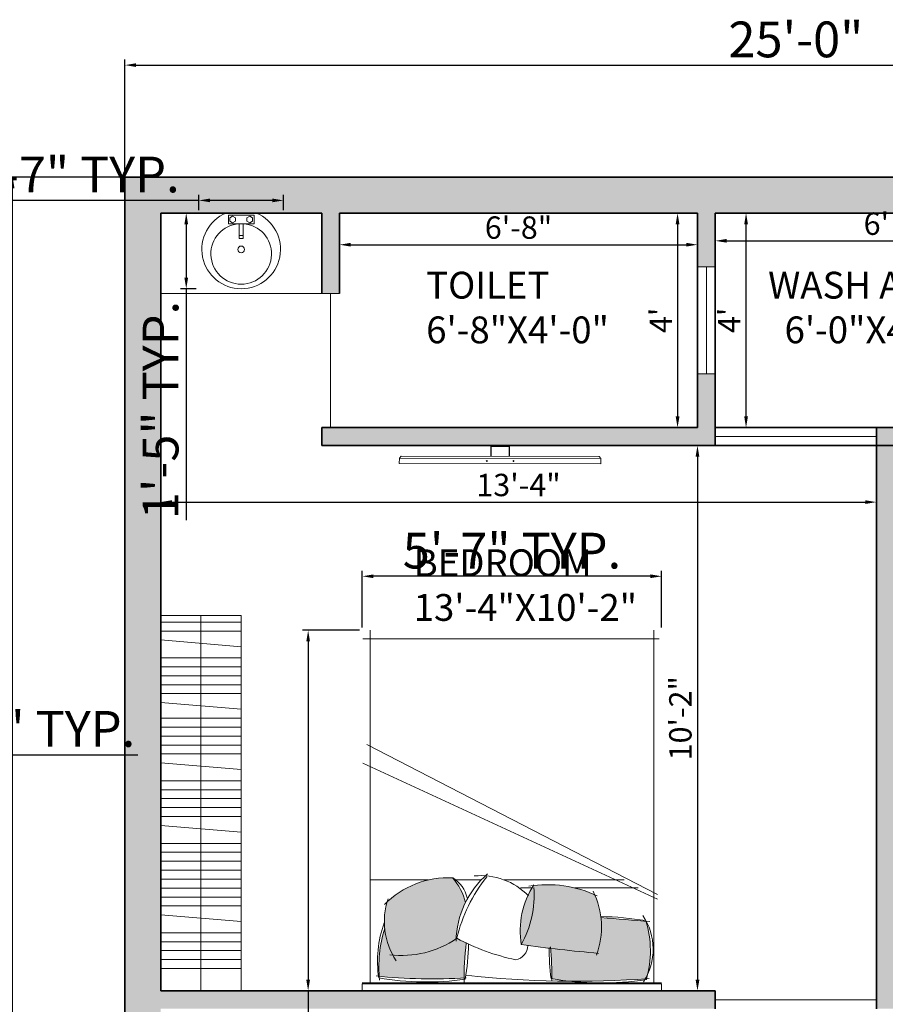
# Model space of a CAD drawing. Units: inches. Extents: x 3259 to 4981, y 1402 to 2026.
# Tile 6 of 11: x 3644 to 3838, y 1722 to 1942. Entities that reach past the tile are written whole.
import ezdxf

# ---------------------------------------------------------------- set-up
doc = ezdxf.new("R2010")
doc.units = ezdxf.units.IN
for name, color, linetype, lineweight in [('0.10', 252, 'Continuous', 9), ('A-ANNO-DIMS', 2, 'Continuous', 13), ('A-AREA-IDEN', 7, 'Continuous', 18), ('A-DOOR', 3, 'Continuous', 18), ('A-EQPM', 8, 'Continuous', 18), ('A-FLOR-CASE', 8, 'Continuous', 18), ('A-FLOR-FIXT', 9, 'Continuous', 18), ('A-FURN', 8, 'Continuous', 13), ('A-GLAZ', 4, 'Continuous', 18), ('A-WALL', 7, 'Continuous', 35), ('A-WALL-PATT', 252, 'Continuous', 13)]:
    doc.layers.add(name, color=color, linetype=linetype, lineweight=lineweight)
doc.layers.add('A-FURN-PATT', color=116, linetype='Continuous', lineweight=13, true_color=0x136734)
doc.styles.get("Standard").update_dxf_attribs({"font": 'arial.ttf'})
doc.dimstyles.new('ISO-25', dxfattribs={"dimtxt": 8, "dimasz": 2.5, "dimexe": 1.25, "dimexo": 0.625, "dimtad": 1, "dimdec": 1, "dimlunit": 3, "dimtxsty": 'Standard', "dimcen": 2.5, "dimclrd": 4, "dimclre": 4, "dimclrt": 1, "dimadec": 0, "dimazin": 0, "dimtfac": 1, "dimtdec": 1, "dimtmove": 0, "dimatfit": 3, "dimfxl": 1, "dimarcsym": 0})

# ---------------------------------------------------------------- blocks, each defined once
blk = doc.blocks.new('camita')
at = {"layer": '0.10'}
for p, q in [((-0.85, -0.045), (0.85, -0.045)), ((-0.805, -0.045), (-0.805, -2.0485)), ((0.805, -0.045), (0.805, -2.0485)), ((-0.8271, -0.521), (0.8464, -1.2932)), ((-0.8271, -0.5476), (0.8236, -1.3992)), ((-0.7161, -0.585), (-0.3554, -0.585)), ((-0.1136, -0.585), (-0.0485, -0.585)), ((-0.638, -0.63), (0.0434, -0.63)), ((0.1749, -0.63), (0.3179, -0.63)), ((0.4739, -0.63), (0.805, -0.63)), ((-0.8354, -2), (0.8464, -2))]:
    blk.add_line(p, q, dxfattribs=at)
blk.add_lwpolyline([(-0.85, -0.0405), (0.85, -0.0405), (0.85, 0), (-0.85, 0)], close=True, dxfattribs=at)
for centre, radius, start, end in [((-0.4574, -0.2364), 0.3443, 147.51, 213.8336), ((-0.3639, -5.8457), 5.7909, 83.80731, 94.12107), ((-0.5104, -1.7232), 1.6781, 80.1255, 98.6619), ((-1.4396, -0.0609), 1.7117, 352.9291, 0.3959), ((0.4863, -1.6286), 1.5781, 80.1602, 98.06), ((-0.1997, -0.2266), 0.5864, 163.9263, 197.1409), ((2.3534, -0.0532), 2.5803, 180.1063, 184.3854), ((-1.5443, -0.2452), 1.3333, 359.9394, 7.5533), ((1.5815, -0.2893), 1.3353, 170.3802, 178.9914), ((0.4524, -3.0675), 2.9996, 83.9026, 93.6759), ((0.0294, -0.1377), 0.7262, 342.5841, 6.0048), ((0.1326, -0.1696), 0.6307, 339.923, 8.7433), ((-0.0543, -0.3633), 0.4542, 159.3026, 206.5026), ((-1.3301, -9.6748), 9.4985, 82.27078, 84.93989), ((-0.007, -0.258), 0.0828, 100.018, 179.736), ((-0.2931, -1.4378), 1.2903, 61.9749, 77.8435), ((0.6265, -0.7518), 0.5508, 82.9691, 124.6739), ((0.3203, -0.3944), 0.4043, 341.4524, 33.4512), ((0.4585, -0.5454), 0.5842, 151.0456, 184.1497), ((-0.5341, -0.3393), 0.4875, 327.2644, 9.0473), ((-0.1986, -0.2742), 0.5159, 310.7395, 359.0576), ((-0.5673, -0.0868), 0.9057, 321.6953, 346.4626), ((-1.8672, -14.986), 14.6323, 84.65974, 85.75157), ((-0.4598, 1.4861), 1.9092, 260.953, 268.6517), ((0.5707, -0.4317), 0.3145, 192.9388, 221.9636), ((0.3612, -0.133), 0.5096, 267.2589, 315.2997), ((-0.2002, 0.064), 0.6673, 244.7809, 279.0606), ((0.179, -0.272), 0.3828, 224.5284, 275.2229), ((0.4384, -0.4834), 0.1898, 193.6849, 236.7035)]:
    blk.add_arc(centre, radius, start, end, dxfattribs=at)
blk = doc.blocks.new('M_BATH_BASIN_Basin - Oval_P')
at = {"color": 0, "linetype": 'ByBlock', "lineweight": -2}
blk.add_lwpolyline([(0, 89.5, -5.027337), (0, -89.5)], format="xyb", close=True, dxfattribs=at)
blk.add_lwpolyline([(63.2, 12, -30), (63.2, -12, -1.097889)], format="xyb", dxfattribs=at)
for points in [[(13.2, -76.2), (13.2, 76.2), (63.2, 76.2), (63.2, -76.2)], [(19.1, 50.8), (28.7, 67.3), (47.7, 67.3), (57.2, 50.8), (47.7, 34.3), (28.7, 34.3)]]:
    blk.add_lwpolyline(points, close=True, dxfattribs=at)
for points in [[(63.2, 12), (151.6, 12), (151.6, -12), (63.2, -12)], [(134.3, 12), (134.3, -12)], [(28.7, -34.3), (47.7, -34.3), (57.2, -50.8), (47.7, -67.3), (28.7, -67.3), (19.1, -50.8), (28.7, -34.3)]]:
    blk.add_lwpolyline(points, dxfattribs=at)
blk.add_circle((216.2, 0), 20.1, dxfattribs=at)
at = {"layer": 'Defpoints'}
for p in [(0, 234), (0, -234)]:
    blk.add_point(p, dxfattribs=at)
blk = doc.blocks.new('*D41')
at = {"layer": 'A-ANNO-DIMS', "color": 0, "lineweight": -2, "transparency": 16777216}
for p, q in [((3715.66, 1898.49), (3715.66, 1890.79)), ((3795.66, 1898.49), (3795.66, 1890.79)), ((3718.16, 1892.04), (3793.16, 1892.04))]:
    blk.add_line(p, q, dxfattribs=at)
at = {"layer": 'A-ANNO-DIMS', "color": 0, "transparency": 16777216}
for points in [[(3718.16, 1892.46), (3718.16, 1891.63), (3715.66, 1892.04)], [(3793.16, 1892.46), (3793.16, 1891.63), (3795.66, 1892.04)]]:
    blk.add_solid(points, dxfattribs=at)
at = {"layer": 'Defpoints', "color": 0, "transparency": 16777216}
for p in [(3715.66, 1899.12), (3795.66, 1899.12), (3795.66, 1892.04)]:
    blk.add_point(p, dxfattribs=at)
at = {"layer": 'A-ANNO-DIMS', "color": 0, "transparency": 16777216, "insert": (3755.66, 1895.22), "char_height": 5, "attachment_point": 5}
blk.add_mtext('6\'-8"', dxfattribs=at)
blk = doc.blocks.new('*D42')
at = {"layer": 'A-ANNO-DIMS', "color": 0, "lineweight": -2, "transparency": 16777216}
for p, q in [((3795.04, 1899.12), (3789.97, 1899.12)), ((3791.22, 1896.62), (3791.22, 1853.62)), ((3795.04, 1851.12), (3789.97, 1851.12))]:
    blk.add_line(p, q, dxfattribs=at)
at = {"layer": 'A-ANNO-DIMS', "color": 0, "transparency": 16777216}
for points in [[(3790.8, 1896.62), (3791.64, 1896.62), (3791.22, 1899.12)], [(3790.8, 1853.62), (3791.64, 1853.62), (3791.22, 1851.12)]]:
    blk.add_solid(points, dxfattribs=at)
at = {"layer": 'Defpoints', "color": 0, "transparency": 16777216}
for p in [(3795.66, 1899.12), (3791.22, 1851.12), (3795.66, 1851.12)]:
    blk.add_point(p, dxfattribs=at)
at = {"layer": 'A-ANNO-DIMS', "color": 0, "transparency": 16777216, "insert": (3788.1, 1875.12), "char_height": 5, "attachment_point": 5, "rotation": 90}
blk.add_mtext("4'", dxfattribs=at)
blk = doc.blocks.new('*D43')
at = {"layer": 'A-ANNO-DIMS', "color": 0, "lineweight": -2, "transparency": 16777216}
for p, q in [((3800.29, 1899.12), (3807.78, 1899.12)), ((3806.53, 1853.62), (3806.53, 1896.62)), ((3800.29, 1851.12), (3807.78, 1851.12))]:
    blk.add_line(p, q, dxfattribs=at)
at = {"layer": 'A-ANNO-DIMS', "color": 0, "transparency": 16777216}
for points in [[(3806.12, 1896.62), (3806.95, 1896.62), (3806.53, 1899.12)], [(3806.12, 1853.62), (3806.95, 1853.62), (3806.53, 1851.12)]]:
    blk.add_solid(points, dxfattribs=at)
at = {"layer": 'Defpoints', "color": 0, "transparency": 16777216}
for p in [(3799.66, 1899.12), (3806.53, 1899.12), (3799.66, 1851.12)]:
    blk.add_point(p, dxfattribs=at)
at = {"layer": 'A-ANNO-DIMS', "color": 0, "transparency": 16777216, "insert": (3803.41, 1875.12), "char_height": 5, "attachment_point": 5, "rotation": 90}
blk.add_mtext("4'", dxfattribs=at)
blk = doc.blocks.new('*D44')
at = {"layer": 'A-ANNO-DIMS', "color": 0, "lineweight": -2, "transparency": 16777216}
for p, q in [((3799.66, 1898.49), (3799.66, 1891.66)), ((3871.66, 1898.49), (3871.66, 1891.66)), ((3802.16, 1892.91), (3869.16, 1892.91))]:
    blk.add_line(p, q, dxfattribs=at)
at = {"layer": 'A-ANNO-DIMS', "color": 0, "transparency": 16777216}
for points in [[(3802.16, 1893.33), (3802.16, 1892.5), (3799.66, 1892.91)], [(3869.16, 1893.33), (3869.16, 1892.5), (3871.66, 1892.91)]]:
    blk.add_solid(points, dxfattribs=at)
at = {"layer": 'Defpoints', "color": 0, "transparency": 16777216}
for p in [(3799.66, 1899.12), (3871.66, 1899.12), (3871.66, 1892.91)]:
    blk.add_point(p, dxfattribs=at)
at = {"layer": 'A-ANNO-DIMS', "color": 0, "transparency": 16777216, "insert": (3835.66, 1896.09), "char_height": 5, "attachment_point": 5}
blk.add_mtext("6'", dxfattribs=at)
blk = doc.blocks.new('*D47')
at = {"layer": 'A-ANNO-DIMS', "color": 0, "lineweight": -2, "transparency": 16777216}
for p, q in [((3675.66, 1843.36), (3675.66, 1833.21)), ((3835.66, 1843.36), (3835.66, 1833.21)), ((3678.16, 1834.46), (3833.16, 1834.46))]:
    blk.add_line(p, q, dxfattribs=at)
at = {"layer": 'A-ANNO-DIMS', "color": 0, "transparency": 16777216}
for points in [[(3678.16, 1834.88), (3678.16, 1834.04), (3675.66, 1834.46)], [(3833.16, 1834.88), (3833.16, 1834.04), (3835.66, 1834.46)]]:
    blk.add_solid(points, dxfattribs=at)
at = {"layer": 'Defpoints', "color": 0, "transparency": 16777216}
for p in [(3675.66, 1843.99), (3835.66, 1843.99), (3835.66, 1834.46)]:
    blk.add_point(p, dxfattribs=at)
at = {"layer": 'A-ANNO-DIMS', "color": 0, "transparency": 16777216, "insert": (3755.66, 1837.64), "char_height": 5, "attachment_point": 5}
blk.add_mtext('13\'-4"', dxfattribs=at)
blk = doc.blocks.new('*D48')
at = {"layer": 'A-ANNO-DIMS', "color": 0, "lineweight": -2, "transparency": 16777216}
for p, q in [((3799.04, 1847.12), (3794.42, 1847.12)), ((3795.67, 1844.62), (3795.67, 1727.62)), ((3799.04, 1725.12), (3794.42, 1725.12))]:
    blk.add_line(p, q, dxfattribs=at)
at = {"layer": 'A-ANNO-DIMS', "color": 0, "transparency": 16777216}
for points in [[(3795.25, 1844.62), (3796.09, 1844.62), (3795.67, 1847.12)], [(3795.25, 1727.62), (3796.09, 1727.62), (3795.67, 1725.12)]]:
    blk.add_solid(points, dxfattribs=at)
at = {"layer": 'Defpoints', "color": 0, "transparency": 16777216}
for p in [(3799.66, 1847.12), (3795.67, 1725.12), (3799.66, 1725.12)]:
    blk.add_point(p, dxfattribs=at)
at = {"layer": 'A-ANNO-DIMS', "color": 0, "transparency": 16777216, "insert": (3792.49, 1786.12), "char_height": 5, "attachment_point": 5, "rotation": 90}
blk.add_mtext('10\'-2"', dxfattribs=at)
blk = doc.blocks.new('WARDROBE-84IN')
for p, q in [((0, 84), (18, 84)), ((9, 0), (9, 84)), ((18, 0), (18, 84)), ((18, 82.5), (0, 82.5)), ((18, 80.5), (0, 80.5)), ((18, 77), (0, 78.5)), ((18, 74.5), (0, 74.5)), ((18, 72.5), (0, 72.5)), ((18, 70.5), (0, 70.5)), ((18, 68.5), (0, 68.5)), ((18, 66.5), (0, 66.5)), ((18, 63), (0, 64.5)), ((18, 61), (0, 61)), ((18, 59), (0, 59)), ((18, 57), (0, 57)), ((18, 55), (0, 55)), ((18, 53), (0, 53)), ((18, 49.5), (0, 51)), ((18, 47), (0, 47)), ((18, 45), (0, 45)), ((18, 43), (0, 43)), ((18, 41), (0, 41)), ((18, 39), (0, 39)), ((18, 35.5), (0, 37)), ((18, 33), (0, 33)), ((18, 31), (0, 31)), ((18, 29), (0, 29)), ((18, 27), (0, 27)), ((18, 25), (0, 25)), ((18, 23), (0, 23)), ((18, 21), (0, 21)), ((18, 19), (0, 19)), ((18, 15.5), (0, 17)), ((18, 13), (0, 13)), ((18, 11), (0, 11)), ((18, 9), (0, 9)), ((18, 7), (0, 7)), ((18, 5), (0, 5))]:
    blk.add_line(p, q)
blk = doc.blocks.new('*D150')
at = {"layer": 'A-ANNO-DIMS', "color": 4, "lineweight": -2, "transparency": 16777216}
for p, q in [((3684.21, 1899.74), (3684.21, 1903.2)), ((3703.12, 1899.74), (3703.12, 1903.2)), ((3684.21, 1901.95), (3595.41, 1901.95)), ((3700.62, 1901.95), (3686.71, 1901.95))]:
    blk.add_line(p, q, dxfattribs=at)
at = {"layer": 'A-ANNO-DIMS', "color": 4, "transparency": 16777216}
for points in [[(3686.71, 1902.37), (3686.71, 1901.54), (3684.21, 1901.95)], [(3700.62, 1902.37), (3700.62, 1901.54), (3703.12, 1901.95)]]:
    blk.add_solid(points, dxfattribs=at)
at = {"layer": 'Defpoints', "color": 0, "transparency": 16777216}
for p in [(3684.21, 1901.95), (3684.21, 1899.12), (3703.12, 1899.12)]:
    blk.add_point(p, dxfattribs=at)
at = {"layer": 'A-ANNO-DIMS', "color": 1, "transparency": 16777216, "insert": (3638.56, 1906.71), "char_height": 8, "attachment_point": 5}
blk.add_mtext('BASIN 1\'-7" TYP.', dxfattribs=at)
blk = doc.blocks.new('*D151')
at = {"layer": 'A-ANNO-DIMS', "color": 4, "lineweight": -2, "transparency": 16777216}
for p, q in [((3683.59, 1899.12), (3680.12, 1899.12)), ((3681.37, 1896.62), (3681.37, 1884.68)), ((3683.59, 1882.18), (3680.12, 1882.18)), ((3681.37, 1882.18), (3681.37, 1830.42))]:
    blk.add_line(p, q, dxfattribs=at)
at = {"layer": 'A-ANNO-DIMS', "color": 4, "transparency": 16777216}
for points in [[(3680.96, 1896.62), (3681.79, 1896.62), (3681.37, 1899.12)], [(3680.96, 1884.68), (3681.79, 1884.68), (3681.37, 1882.18)]]:
    blk.add_solid(points, dxfattribs=at)
at = {"layer": 'Defpoints', "color": 0, "transparency": 16777216}
for p in [(3684.21, 1899.12), (3681.37, 1882.18), (3684.21, 1882.18)]:
    blk.add_point(p, dxfattribs=at)
at = {"layer": 'A-ANNO-DIMS', "color": 1, "transparency": 16777216, "insert": (3676.66, 1855.05), "char_height": 8, "attachment_point": 5, "rotation": 90}
blk.add_mtext('1\'-5" TYP.', dxfattribs=at)
blk = doc.blocks.new('*D157')
at = {"layer": 'A-ANNO-DIMS', "color": 4, "lineweight": -2, "transparency": 16777216}
for p, q in [((3546.53, 1766.36), (3546.53, 1779.18)), ((3549.03, 1777.93), (3590.67, 1777.93)), ((3593.17, 1766.36), (3593.17, 1779.18)), ((3593.17, 1777.93), (3670.53, 1777.93))]:
    blk.add_line(p, q, dxfattribs=at)
at = {"layer": 'A-ANNO-DIMS', "color": 4, "transparency": 16777216}
for points in [[(3549.03, 1778.35), (3549.03, 1777.51), (3546.53, 1777.93)], [(3590.67, 1778.35), (3590.67, 1777.51), (3593.17, 1777.93)]]:
    blk.add_solid(points, dxfattribs=at)
at = {"layer": 'Defpoints', "color": 0, "transparency": 16777216}
for p in [(3593.17, 1777.93), (3546.53, 1765.74), (3593.17, 1765.74)]:
    blk.add_point(p, dxfattribs=at)
at = {"layer": 'A-ANNO-DIMS', "color": 1, "transparency": 16777216, "insert": (3633.1, 1782.69), "char_height": 8, "attachment_point": 5}
blk.add_mtext('3\'-10 1/2" TYP.', dxfattribs=at)
blk = doc.blocks.new('*D158')
at = {"layer": 'A-ANNO-DIMS', "color": 4, "lineweight": -2, "transparency": 16777216}
for p, q in [((3720.1, 1805.78), (3707.38, 1805.78)), ((3708.63, 1803.28), (3708.63, 1727.62)), ((3720.1, 1725.12), (3707.38, 1725.12)), ((3708.63, 1725.12), (3708.63, 1628.23))]:
    blk.add_line(p, q, dxfattribs=at)
at = {"layer": 'A-ANNO-DIMS', "color": 4, "transparency": 16777216}
for points in [[(3708.21, 1803.28), (3709.04, 1803.28), (3708.63, 1805.78)], [(3708.21, 1727.62), (3709.04, 1727.62), (3708.63, 1725.12)]]:
    blk.add_solid(points, dxfattribs=at)
at = {"layer": 'Defpoints', "color": 0, "transparency": 16777216}
for p in [(3720.73, 1805.78), (3708.63, 1725.12), (3720.73, 1725.12)]:
    blk.add_point(p, dxfattribs=at)
at = {"layer": 'A-ANNO-DIMS', "color": 1, "transparency": 16777216, "insert": (3703.87, 1675.42), "char_height": 8, "attachment_point": 5, "rotation": 90}
blk.add_mtext('BED 6\'-8 1/2" TYP.', dxfattribs=at)
blk = doc.blocks.new('*D159')
at = {"layer": 'A-ANNO-DIMS', "color": 4, "lineweight": -2, "transparency": 16777216}
for p, q in [((3720.73, 1806.4), (3720.73, 1819.12)), ((3785.16, 1817.87), (3723.23, 1817.87)), ((3787.66, 1806.4), (3787.66, 1819.12))]:
    blk.add_line(p, q, dxfattribs=at)
at = {"layer": 'A-ANNO-DIMS', "color": 4, "transparency": 16777216}
for points in [[(3723.23, 1818.29), (3723.23, 1817.46), (3720.73, 1817.87)], [(3785.16, 1818.29), (3785.16, 1817.46), (3787.66, 1817.87)]]:
    blk.add_solid(points, dxfattribs=at)
at = {"layer": 'Defpoints', "color": 0, "transparency": 16777216}
for p in [(3720.73, 1817.87), (3720.73, 1805.78), (3787.66, 1805.78)]:
    blk.add_point(p, dxfattribs=at)
at = {"layer": 'A-ANNO-DIMS', "color": 1, "transparency": 16777216, "insert": (3754.19, 1822.57), "char_height": 8, "attachment_point": 5}
blk.add_mtext('5\'-7" TYP.', dxfattribs=at)
blk = doc.blocks.new('*D186')
at = {"layer": 'A-ANNO-DIMS', "color": 4, "lineweight": -2, "transparency": 16777216}
for p, q in [((3667.66, 1907.74), (3667.66, 1933.47)), ((3670.16, 1932.22), (3965.16, 1932.22)), ((3967.66, 1907.74), (3967.66, 1933.47))]:
    blk.add_line(p, q, dxfattribs=at)
at = {"layer": 'A-ANNO-DIMS', "color": 4, "transparency": 16777216}
for points in [[(3670.16, 1932.63), (3670.16, 1931.8), (3667.66, 1932.22)], [(3965.16, 1932.63), (3965.16, 1931.8), (3967.66, 1932.22)]]:
    blk.add_solid(points, dxfattribs=at)
at = {"layer": 'Defpoints', "color": 0, "transparency": 16777216}
for p in [(3967.66, 1932.22), (3667.66, 1907.12), (3967.66, 1907.12)]:
    blk.add_point(p, dxfattribs=at)
at = {"layer": 'A-ANNO-DIMS', "color": 1, "transparency": 16777216, "insert": (3817.66, 1936.93), "char_height": 8, "attachment_point": 5}
blk.add_mtext('25\'-0"', dxfattribs=at)
blk = doc.blocks.new('*D187')
at = {"layer": 'A-ANNO-DIMS', "color": 4, "lineweight": -2, "transparency": 16777216}
for p, q in [((3667.04, 1907.12), (3641.31, 1907.12)), ((3642.56, 1477.62), (3642.56, 1904.62)), ((3667.04, 1475.12), (3641.31, 1475.12))]:
    blk.add_line(p, q, dxfattribs=at)
at = {"layer": 'A-ANNO-DIMS', "color": 4, "transparency": 16777216}
for points in [[(3642.15, 1904.62), (3642.98, 1904.62), (3642.56, 1907.12)], [(3642.15, 1477.62), (3642.98, 1477.62), (3642.56, 1475.12)]]:
    blk.add_solid(points, dxfattribs=at)
at = {"layer": 'Defpoints', "color": 0, "transparency": 16777216}
for p in [(3642.56, 1907.12), (3667.66, 1907.12), (3667.66, 1475.12)]:
    blk.add_point(p, dxfattribs=at)
at = {"layer": 'A-ANNO-DIMS', "color": 1, "transparency": 16777216, "insert": (3637.85, 1691.12), "char_height": 8, "attachment_point": 5, "rotation": 90}
blk.add_mtext('36\'-0"', dxfattribs=at)

msp = doc.modelspace()

# ---------------------------------------------------------------- hatches: boundary and pattern name
at = {"layer": 'A-FURN-PATT'}
h = msp.add_hatch(color=256, dxfattribs=at)
h.dxf.hatch_style = 1
h.paths.add_polyline_path([(3758.97, 1748.69, 0.181694), (3756.27, 1735.46, 0.011408), (3773.23, 1733.55, 0.189536), (3772.7, 1746.63, 0.134508)])
h.paths.add_polyline_path([(3741.72, 1736.79, -0.104045), (3743.79, 1744.89, 0.127326), (3740.93, 1750.4, 0.202559), (3726.27, 1745.01, 0.194952), (3727.55, 1733.12, 0.173835)])
h = msp.add_hatch(color=256, dxfattribs=at)
h.dxf.hatch_style = 1
h.paths.add_polyline_path([(3774.09, 1741.55, -0.113891), (3773.23, 1733.55, -0.006967), (3762.86, 1734.62, -0.016701), (3763.13, 1727.84, 0.015442), (3767.17, 1727.28, 0.01851), (3784.04, 1727.8, 0.020657), (3784.54, 1728.8, 0.131047), (3784.17, 1740.69, -0.004387)])
h.paths.add_polyline_path([(3743.99, 1735.81, -0.011742), (3741.86, 1736.88, -0.175864), (3727.55, 1733.12, -0.098488), (3725.74, 1739.06, 0.094792), (3724.52, 1728.39, 0.040212), (3743.48, 1728, -0.029051)])
at = {"layer": 'A-WALL-PATT'}
h = msp.add_hatch(color=256, dxfattribs=at)
h.dxf.hatch_style = 1
h.paths.add_polyline_path([(3839.66, 1851.12), (3835.66, 1851.12), (3835.66, 1721.12), (3839.66, 1721.12), (3839.66, 1777.43), (3839.65, 1777.43), (3839.65, 1777.47), (3839.66, 1777.47), (3839.66, 1781.5), (3839.66, 1781.5), (3839.66, 1781.55)], flags=17)
h.paths.add_polyline_path([(3799.66, 1863.12), (3795.66, 1863.12), (3795.66, 1851.12), (3711.66, 1851.12), (3711.66, 1847.12), (3749.49, 1847.12), (3749.49, 1847.13), (3749.54, 1847.13), (3749.54, 1847.12), (3753.57, 1847.12), (3753.57, 1847.12), (3753.61, 1847.12), (3799.66, 1847.12)], flags=17)
h.paths.add_polyline_path([(3875.66, 1863.12), (3871.66, 1863.12), (3871.66, 1847.12), (3875.66, 1847.12)], flags=17)
h.paths.add_polyline_path([(3967.66, 1907.12), (3667.66, 1907.12), (3667.66, 1579.12), (3839.66, 1579.12), (3839.66, 1587.12), (3835.66, 1587.12), (3835.66, 1583.12), (3675.66, 1583.12), (3675.66, 1721.12), (3799.66, 1721.12), (3799.66, 1725.12), (3675.66, 1725.12), (3675.66, 1899.12), (3711.66, 1899.12), (3711.66, 1881.12), (3715.66, 1881.12), (3715.66, 1899.12), (3795.66, 1899.12), (3795.66, 1887.12), (3799.66, 1887.12), (3799.66, 1899.12), (3871.66, 1899.12), (3871.66, 1887.12), (3875.66, 1887.12), (3875.66, 1899.12), (3959.66, 1899.12), (3959.66, 1851.12), (3905.66, 1851.12), (3905.66, 1847.12), (3959.66, 1847.12), (3959.66, 1643.12), (3941.66, 1643.12), (3941.66, 1639.12), (3967.66, 1639.12)])
h.paths.add_polyline_path([(3839.66, 1667.12), (3835.66, 1667.12), (3835.66, 1635.12), (3839.66, 1635.12), (3839.66, 1639.12), (3857.66, 1639.12), (3857.66, 1643.12), (3839.66, 1643.12)], flags=17)

# ---------------------------------------------------------------- linework, layer by layer
at = {"layer": 'A-DOOR'}
for p, q in [((3713.66, 1881.12), (3713.66, 1851.12)), ((3799.66, 1723.12), (3835.66, 1723.12))]:
    msp.add_line(p, q, dxfattribs=at)
at = {"layer": 'A-EQPM'}
for p, q in [((3749.49, 1847.13), (3749.49, 1844.73)), ((3749.49, 1847.13), (3749.54, 1847.13)), ((3749.54, 1847.13), (3749.53, 1844.73)), ((3749.54, 1846.89), (3753.56, 1846.88)), ((3753.57, 1847.12), (3753.56, 1844.72)), ((3753.57, 1847.12), (3753.61, 1847.12)), ((3753.61, 1847.12), (3753.61, 1844.72)), ((3729.02, 1844.29), (3729.42, 1844.77)), ((3729.42, 1844.77), (3773.67, 1844.68)), ((3774.08, 1844.2), (3773.67, 1844.68))]:
    msp.add_line(p, q, dxfattribs=at)
msp.add_lwpolyline([(3729.01, 1843.09), (3774.07, 1843), (3774.08, 1844.2), (3729.02, 1844.29), (3729.01, 1843.09)], dxfattribs=at)
for centre in [(3748.55, 1843.65), (3754.54, 1843.64)]:
    msp.add_circle(centre, 0.0959, dxfattribs=at)
at = {"layer": 'A-FLOR-CASE'}
msp.add_line((3675.66, 1881.12), (3715.66, 1881.12), dxfattribs=at)
at = {"layer": 'A-GLAZ'}
for p, q in [((3795.66, 1887.12), (3799.66, 1887.12)), ((3797.66, 1887.12), (3797.66, 1863.12)), ((3795.66, 1863.12), (3799.66, 1863.12)), ((3799.66, 1849.12), (3835.66, 1849.12))]:
    msp.add_line(p, q, dxfattribs=at)
at = {"layer": 'A-WALL'}
for p, q in [((3675.66, 1899.12), (3711.66, 1899.12)), ((3675.66, 1725.12), (3675.66, 1899.12)), ((3711.66, 1899.12), (3711.66, 1881.12)), ((3715.66, 1899.12), (3795.66, 1899.12)), ((3715.66, 1899.12), (3715.66, 1881.12)), ((3795.66, 1899.12), (3795.66, 1851.12)), ((3799.66, 1899.12), (3871.66, 1899.12)), ((3799.66, 1899.12), (3799.66, 1847.12)), ((3711.66, 1851.12), (3795.66, 1851.12)), ((3711.66, 1851.12), (3711.66, 1847.12)), ((3799.66, 1851.12), (3871.66, 1851.12)), ((3835.66, 1721.12), (3835.66, 1851.12)), ((3711.66, 1847.12), (3871.66, 1847.12)), ((3675.66, 1725.12), (3799.66, 1725.12)), ((3799.66, 1721.12), (3799.66, 1725.12))]:
    msp.add_line(p, q, dxfattribs=at)
msp.add_lwpolyline([(3959.66, 1475.12), (3667.66, 1475.12), (3667.66, 1907.12), (3967.66, 1907.12), (3967.66, 1475.12), (3959.66, 1475.12)], dxfattribs=at)

# ---------------------------------------------------------------- block references
at = {"layer": 'A-FLOR-CASE'}
msp.add_blockref('WARDROBE-84IN', (3675.66, 1725.12), dxfattribs=at)
at = {"layer": 'A-FLOR-FIXT', "xscale": -0.0376189459335944, "yscale": 0.0376189459335944, "zscale": 0.0376189459335944, "rotation": 90}
msp.add_blockref('M_BATH_BASIN_Basin - Oval_P', (3693.66, 1899.12), dxfattribs=at)
at = {"layer": 'A-FURN', "xscale": 39.375, "yscale": 39.375, "zscale": 39.375, "rotation": 180}
msp.add_blockref('camita', (3754.19, 1725.12), dxfattribs=at)

# ---------------------------------------------------------------- texts
at = {"layer": 'A-AREA-IDEN', "char_height": 6, "attachment_point": 1}
for s, width, insert in [('TOILET\\P6\'-8"X4\'-0"', 127.3061, (3735.02, 1885.99)), ('WASH AREA\\P  6\'-0"X4\'-0"', 127.3061, (3811.47, 1885.99)), ('BEDROOM\\P13\'-4"X10\'-2"', 86.9528, (3732.22, 1823.9))]:
    msp.add_mtext_dynamic_manual_height_columns(s, width=width, gutter_width=12.5, heights=[0], dxfattribs=dict(at, insert=insert))

# ---------------------------------------------------------------- dimensions: what is measured, and where the dimension line sits
at = {"layer": 'A-ANNO-DIMS'}
for base, p1, p2, override, picture, middle in [((3967.66, 1932.22), (3667.66, 1907.12), (3967.66, 1907.12), {"dimdec": 1, "dimlfac": 1, "dimrnd": 0, "dimzin": 1, "dimdsep": 46, "dimlunit": 4, "dimfrac": 2}, '*D186', (3817.66, 1936.93)), ((3795.66, 1892.04), (3715.66, 1899.12), (3795.66, 1899.12), {"dimtxt": 5, "dimclrd": 0, "dimclre": 0, "dimclrt": 0}, '*D41', (3755.66, 1895.22)), ((3871.66, 1892.91), (3799.66, 1899.12), (3871.66, 1899.12), {"dimtxt": 5, "dimclrd": 0, "dimclre": 0, "dimclrt": 0}, '*D44', (3835.66, 1896.09)), ((3835.66, 1834.46), (3675.66, 1843.99), (3835.66, 1843.99), {"dimtxt": 5, "dimclrd": 0, "dimclre": 0, "dimclrt": 0}, '*D47', (3755.66, 1837.64))]:
    dim = msp.add_linear_dim(base=base, p1=p1, p2=p2, dimstyle='ISO-25', override=override, dxfattribs=at)
    dim.commit()
    dim.dimension.update_dxf_attribs({"geometry": picture, "text_midpoint": middle})
for base, p1, p2, angle, text, picture, middle in [((3684.21, 1901.95), (3703.12, 1899.12), (3684.21, 1899.12), 180, 'BASIN <> TYP.', '*D150', (3638.56, 1906.71)), ((3681.37, 1882.18), (3684.21, 1899.12), (3684.21, 1882.18), 270, '<> TYP.', '*D151', (3676.66, 1855.05)), ((3720.73, 1817.87), (3787.66, 1805.78), (3720.73, 1805.78), 180, '<> TYP.', '*D159', (3754.19, 1822.57)), ((3708.63, 1725.12), (3720.73, 1805.78), (3720.73, 1725.12), 270, 'BED <> TYP.', '*D158', (3703.87, 1675.42))]:
    dim = msp.add_linear_dim(base=base, p1=p1, p2=p2, angle=angle, text=text, dimstyle='ISO-25', override={"dimdec": 1, "dimlfac": 1, "dimrnd": 0, "dimzin": 1, "dimdsep": 46, "dimlunit": 4, "dimfrac": 2}, dxfattribs=at)
    dim.commit()
    dim.dimension.update_dxf_attribs({"geometry": picture, "text_midpoint": middle})
for base, p1, p2, override, picture, middle in [((3642.56, 1907.12), (3667.66, 1475.12), (3667.66, 1907.12), {"dimdec": 1, "dimlfac": 1, "dimrnd": 0, "dimzin": 1, "dimdsep": 46, "dimlunit": 4, "dimfrac": 2}, '*D187', (3637.85, 1691.12)), ((3791.22, 1851.12), (3795.66, 1899.12), (3795.66, 1851.12), {"dimtxt": 5, "dimclrd": 0, "dimclre": 0, "dimclrt": 0}, '*D42', (3788.1, 1875.12)), ((3806.53, 1899.12), (3799.66, 1851.12), (3799.66, 1899.12), {"dimtxt": 5, "dimclrd": 0, "dimclre": 0, "dimclrt": 0}, '*D43', (3803.41, 1875.12)), ((3795.67, 1725.12), (3799.66, 1847.12), (3799.66, 1725.12), {"dimtxt": 5, "dimclrd": 0, "dimclre": 0, "dimclrt": 0}, '*D48', (3792.49, 1786.12))]:
    dim = msp.add_linear_dim(base=base, p1=p1, p2=p2, angle=90, dimstyle='ISO-25', override=override, dxfattribs=at)
    dim.commit()
    dim.dimension.update_dxf_attribs({"geometry": picture, "text_midpoint": middle})
dim = msp.add_linear_dim(base=(3593.17, 1777.93), p1=(3546.53, 1765.74), p2=(3593.17, 1765.74), text='<> TYP.', dimstyle='ISO-25', override={"dimdec": 1, "dimlfac": 1, "dimrnd": 0, "dimzin": 1, "dimdsep": 46, "dimlunit": 4, "dimfrac": 2}, dxfattribs=at)
dim.commit()
dim.dimension.update_dxf_attribs({"geometry": '*D157', "text_midpoint": (3633.1, 1782.69)})

doc.saveas('drawing.dxf')
